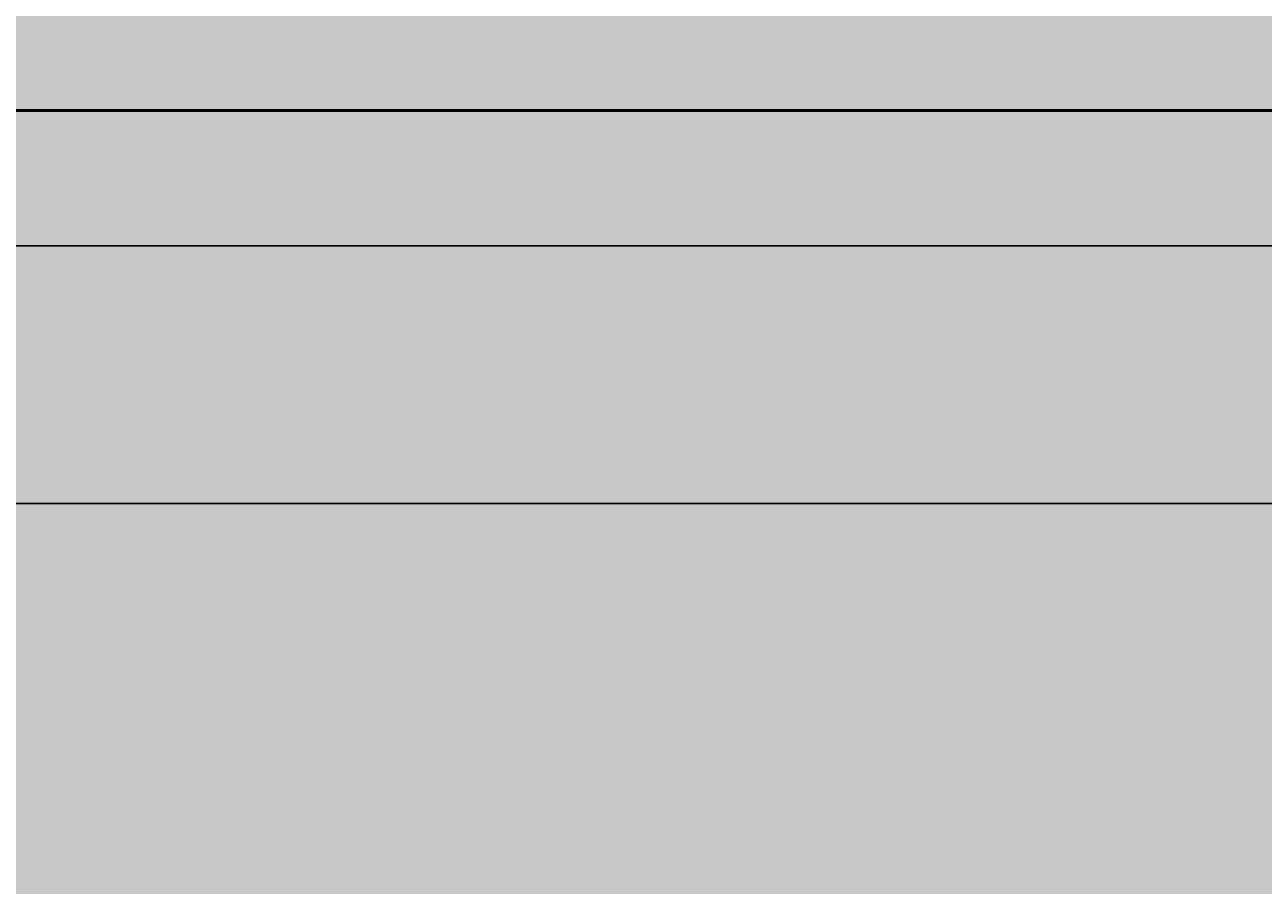
# Model space of a CAD drawing. Units: inches. Extents: x -12 to 334, y -10 to 186.
# Tile 43 of 77: x 175 to 198, y 49 to 65. Entities that reach past the tile are written whole.
import ezdxf
from ezdxf import colors
from ezdxf.entities.mleader import LeaderData, LeaderLine
from ezdxf.math import Vec2, Vec3

# ---------------------------------------------------------------- set-up
doc = ezdxf.new("R2010")
doc.units = ezdxf.units.IN
doc.header["$MEASUREMENT"] = 0
for name, color, linetype, lineweight in [('M-ANNO-TEXT', 3, 'Continuous', 25), ('M-DIMS', 2, 'Continuous', 18), ('M-EQPM', 7, 'Continuous', 50), ('M-EQPM-PATT', 8, 'Continuous', 18)]:
    doc.layers.add(name, color=color, linetype=linetype, lineweight=lineweight)
doc.styles.get("Standard").update_dxf_attribs({"font": 'arial.ttf'})
doc.dimstyles.get("Standard").update_dxf_attribs({"dimtxt": 0.18, "dimasz": 0.18, "dimexe": 0.18, "dimexo": 0.0625, "dimgap": 0.09, "dimtad": 0, "dimtih": 1, "dimtoh": 1, "dimdec": 4, "dimzin": 0, "dimdsep": 46, "dimtxsty": 'Standard', "dimcen": 0.09, "dimadec": 0, "dimazin": 0, "dimtfac": 1, "dimtdec": 4, "dimtofl": 0, "dimtmove": 0, "dimatfit": 3, "dimfxl": 1, "dimtolj": 1, "dimtzin": 0, "dimarcsym": 0})

# ---------------------------------------------------------------- blocks, each defined once
blk = doc.blocks.new('*D1')
at = {"layer": 'Defpoints', "color": 0, "transparency": 16777216}
for p in [(281.426, 91.899), (3.376, 80.692), (281.426, 14.304)]:
    blk.add_point(p, dxfattribs=at)
at = {"layer": 'M-DIMS', "color": 0, "lineweight": -2, "transparency": 16777216}
for p, q in [((281.426, 91.836), (281.426, 14.124)), ((3.376, 80.629), (3.376, 14.124)), ((3.556, 14.304), (141.935, 14.304)), ((281.246, 14.304), (142.867, 14.304))]:
    blk.add_line(p, q, dxfattribs=at)
at = {"layer": 'M-DIMS', "color": 0, "transparency": 16777216}
for points in [[(3.556, 14.334), (3.556, 14.274), (3.376, 14.304)], [(281.246, 14.334), (281.246, 14.274), (281.426, 14.304)]]:
    blk.add_solid(points, dxfattribs=at)
at = {"layer": 'M-DIMS', "color": 0, "transparency": 16777216, "insert": (142.401, 14.304), "char_height": 0.18, "attachment_point": 5}
blk.add_mtext('\\A1;278.05', dxfattribs=at)
blk = doc.blocks.new('*D17')
at = {"layer": 'Defpoints', "color": 0, "transparency": 16777216}
for p in [(106.177, 102.896), (105.892, 56.321), (295.976, 56.321)]:
    blk.add_point(p, dxfattribs=at)
at = {"layer": 'M-DIMS', "color": 0, "lineweight": -2, "transparency": 16777216}
for p, q in [((106.24, 102.896), (296.156, 102.896)), ((295.976, 102.716), (295.976, 79.79)), ((295.976, 56.501), (295.976, 79.426)), ((105.954, 56.321), (296.156, 56.321))]:
    blk.add_line(p, q, dxfattribs=at)
at = {"layer": 'M-DIMS', "color": 0, "transparency": 16777216}
for points in [[(295.946, 102.716), (296.006, 102.716), (295.976, 102.896)], [(295.946, 56.501), (296.006, 56.501), (295.976, 56.321)]]:
    blk.add_solid(points, dxfattribs=at)
at = {"layer": 'M-DIMS', "color": 0, "transparency": 16777216, "insert": (295.976, 79.608), "char_height": 0.18, "attachment_point": 5}
blk.add_mtext('\\A1;46.575', dxfattribs=at)
blk = doc.blocks.new('*D32')
at = {"layer": 'Defpoints', "color": 0, "transparency": 16777216}
for p in [(170.908, 61.105), (216.428, 61.105), (216.428, 14.304)]:
    blk.add_point(p, dxfattribs=at)
at = {"layer": 'M-DIMS', "color": 0, "lineweight": -2, "transparency": 16777216}
for p, q in [((170.908, 61.042), (170.908, 14.124)), ((216.428, 61.042), (216.428, 14.124)), ((171.088, 14.304), (193.271, 14.304)), ((216.248, 14.304), (194.064, 14.304))]:
    blk.add_line(p, q, dxfattribs=at)
at = {"layer": 'M-DIMS', "color": 0, "transparency": 16777216}
for points in [[(171.088, 14.334), (171.088, 14.274), (170.908, 14.304)], [(216.248, 14.334), (216.248, 14.274), (216.428, 14.304)]]:
    blk.add_solid(points, dxfattribs=at)
at = {"layer": 'M-DIMS', "color": 0, "transparency": 16777216, "insert": (193.668, 14.304), "char_height": 0.18, "attachment_point": 5}
blk.add_mtext('\\A1;45.52', dxfattribs=at)
blk = doc.blocks.new('*D35')
at = {"layer": 'Defpoints', "color": 0, "transparency": 16777216}
for p in [(216.428, 98.108), (-11.174, 61.105), (216.428, 61.105)]:
    blk.add_point(p, dxfattribs=at)
at = {"layer": 'M-DIMS', "color": 0, "lineweight": -2, "transparency": 16777216}
for p, q in [((216.365, 98.108), (-11.354, 98.108)), ((-11.174, 97.928), (-11.174, 79.788)), ((-11.174, 61.285), (-11.174, 79.424)), ((216.365, 61.105), (-11.354, 61.105))]:
    blk.add_line(p, q, dxfattribs=at)
at = {"layer": 'M-DIMS', "color": 0, "transparency": 16777216}
for points in [[(-11.204, 97.928), (-11.144, 97.928), (-11.174, 98.108)], [(-11.204, 61.285), (-11.144, 61.285), (-11.174, 61.105)]]:
    blk.add_solid(points, dxfattribs=at)
at = {"layer": 'M-DIMS', "color": 0, "transparency": 16777216, "insert": (-11.174, 79.606), "char_height": 0.18, "attachment_point": 5}
blk.add_mtext('\\A1;37', dxfattribs=at)
blk = doc.blocks.new('*D39')
at = {"layer": 'Defpoints', "color": 0, "transparency": 16777216}
for p in [(279.726, 80.692), (-11.174, 45.854), (269.381, 45.854)]:
    blk.add_point(p, dxfattribs=at)
at = {"layer": 'M-DIMS', "color": 0, "lineweight": -2, "transparency": 16777216}
for p, q in [((279.664, 80.692), (-11.354, 80.692)), ((-11.174, 80.512), (-11.174, 63.455)), ((-11.174, 46.034), (-11.174, 63.091)), ((269.318, 45.854), (-11.354, 45.854))]:
    blk.add_line(p, q, dxfattribs=at)
at = {"layer": 'M-DIMS', "color": 0, "transparency": 16777216}
for points in [[(-11.204, 80.512), (-11.144, 80.512), (-11.174, 80.692)], [(-11.204, 46.034), (-11.144, 46.034), (-11.174, 45.854)]]:
    blk.add_solid(points, dxfattribs=at)
at = {"layer": 'M-DIMS', "color": 0, "transparency": 16777216, "insert": (-11.174, 63.273), "char_height": 0.18, "attachment_point": 5}
blk.add_mtext('\\A1;34.84', dxfattribs=at)
blk = doc.blocks.new('*D41')
at = {"layer": 'Defpoints', "color": 0, "transparency": 16777216}
for p in [(190.169, 91.899), (277.343, 68.515)]:
    blk.add_point(p, dxfattribs=at)
at = {"layer": 'M-DIMS', "color": 0, "lineweight": -2, "transparency": 16777216}
for p, q in [((190.169, 91.809), (190.169, 91.989)), ((190.079, 91.899), (190.259, 91.899)), ((329.648, 54.485), (277.517, 68.469)), ((329.828, 54.485), (329.648, 54.485))]:
    blk.add_line(p, q, dxfattribs=at)
at = {"layer": 'M-DIMS', "color": 0, "transparency": 16777216}
blk.add_solid([(277.525, 68.498), (277.509, 68.44), (277.343, 68.515)], dxfattribs=at)
at = {"layer": 'M-DIMS', "color": 0, "transparency": 16777216, "insert": (330.307, 54.485), "char_height": 0.18, "attachment_point": 5}
blk.add_mtext('\\A1;R90.26', dxfattribs=at)

msp = doc.modelspace()

# ---------------------------------------------------------------- hatches: boundary and pattern name
at = {"layer": 'M-EQPM-PATT'}
h = msp.add_hatch(color=256, dxfattribs=at)
h.set_gradient(color1=(205, 32, 39), color2=(205, 32, 39), tint=1)
h.paths.add_polyline_path([(64.5, 80.754), (64.5, 89.8963), (226.6083, 89.8963, -1), (226.6083, 69.6117), (64.5, 69.6117), (64.5, 78.754), (4.4744, 78.754, 0.384914), (23.5807, 61.4872), (37.1002, 61.4872), (37.1002, 33.6752), (53.1002, 33.6752), (53.1002, 61.4872), (64.5, 61.4872), (64.5, 63.6117), (226.6083, 63.6117, 1), (226.6083, 95.8963), (64.5, 95.8963), (64.5, 99.8958), (53.1002, 99.8958), (53.1002, 127.7078), (37.1002, 127.7078), (37.1002, 99.8958), (23.5807, 99.8958, 0.4132606), (4.3766, 80.754)])
h.paths.add_polyline_path([(64.5, 91.8963), (64.5, 93.8963), (226.6083, 93.8963, -1), (226.6083, 65.6117), (64.5, 65.6117), (64.5, 67.6117), (226.6083, 67.6117, 1), (226.6083, 91.8963)], flags=16)
h = msp.add_hatch(color=256, dxfattribs=at)
h.set_gradient(color1=(94, 103, 175), color2=(94, 103, 175), tint=1)
h.paths.add_polyline_path([(129.093, 89.8963), (86.8879, 89.8963), (86.8879, 69.6117), (129.093, 69.6117)], flags=17)
h.paths.add_polyline_path([(170.9079, 89.8963), (130.8573, 89.8963), (130.8573, 69.6117), (170.9079, 69.6117)], flags=17)
h.paths.add_polyline_path([(216.4278, 89.8963), (172.6722, 89.8963), (172.6722, 69.6117), (216.4278, 69.6117)], flags=17)
h.paths.add_polyline_path([(245.9354, 82.6969), (247.9354, 82.6969), (247.9354, 46.8541), (268.3808, 46.8541, 0.0998398), (279.7263, 80.6915), (251.9801, 80.6915, 0.4142136), (231.7758, 100.8958), (84.7229, 100.8958), (84.7229, 109.0583), (83.7229, 109.0583), (83.7229, 95.8963), (129.093, 95.8963), (129.093, 98.1081), (130.8573, 98.1081), (130.8573, 95.8963), (170.9079, 95.8963), (170.9079, 98.1081), (172.6722, 98.1081), (172.6722, 95.8963), (216.4278, 95.8963), (216.4278, 98.1081), (218.1922, 98.1081), (218.1922, 95.8963), (226.6083, 95.8963, -1), (226.6083, 63.6117), (218.1922, 63.6117), (218.1922, 61.1045), (216.4278, 61.1045), (216.4278, 63.6117), (172.6722, 63.6117), (172.6722, 61.1045), (170.9079, 61.1045), (170.9079, 63.6117), (130.8573, 63.6117), (130.8573, 61.1045), (129.093, 61.1045), (129.093, 63.6117), (87.8879, 63.6117), (87.8879, 56.3205), (105.8919, 56.3205), (105.8919, 28.8541), (115.8919, 28.8541), (115.8919, 46.8541), (222.5761, 46.8541), (222.5761, 30.8541), (232.5761, 30.8541), (232.5761, 46.8541), (245.9354, 46.8541)])
h.paths.add_polyline_path([(86.8879, 89.8963), (75.9244, 89.8963), (75.9244, 69.6117), (86.8879, 69.6117)])
h.paths.add_polyline_path([(83.7229, 109.0583), (75.9244, 109.0583), (75.9244, 95.8963), (83.7229, 95.8963)])
h.paths.add_polyline_path([(226.6083, 89.8963), (218.1922, 89.8963), (218.1922, 69.6117), (226.6083, 69.6117, 1)], flags=17)
h = msp.add_hatch(color=256, dxfattribs=at)
h.set_gradient(color1=(0, 0, 255), color2=(0, 0, 255), tint=1)
h.paths.add_polyline_path([(84.7229, 100.8958), (84.7229, 109.0583), (83.7229, 109.0583), (83.7229, 95.8963), (129.093, 95.8963), (129.093, 98.1081), (130.8573, 98.1081), (130.8573, 95.8963), (170.9079, 95.8963), (170.9079, 98.1081), (172.6722, 98.1081), (172.6722, 95.8963), (216.4278, 95.8963), (216.4278, 98.1081), (218.1922, 98.1081), (218.1922, 95.8963), (226.6083, 95.8963, -1), (226.6083, 63.6117), (218.1922, 63.6117), (218.1922, 61.1045), (216.4278, 61.1045), (216.4278, 63.6117), (172.6722, 63.6117), (172.6722, 61.1045), (170.9079, 61.1045), (170.9079, 63.6117), (130.8573, 63.6117), (130.8573, 61.1045), (129.093, 61.1045), (129.093, 63.6117), (87.8879, 63.6117), (87.8879, 56.3205), (105.8919, 56.3205), (105.8919, 28.8541), (115.8919, 28.8541), (115.8919, 46.8541), (222.5761, 46.8541), (222.5761, 30.8541), (232.5761, 30.8541), (232.5761, 46.8541), (245.9354, 46.8541), (245.9354, 82.6969), (247.9354, 82.6969), (247.9354, 46.8541), (268.3808, 46.8541, 0.0998398), (279.7263, 80.6915), (251.9801, 80.6915, 0.4142136), (231.7758, 100.8958)])

# ---------------------------------------------------------------- linework, layer by layer
at = {"layer": 'M-EQPM'}
msp.add_lwpolyline([(64.5, 63.6117), (226.6083, 63.6117, 1), (226.6083, 95.8963), (64.5, 95.8963)], format="xyb", dxfattribs=at)

# ---------------------------------------------------------------- dimensions: what is measured, and where the dimension line sits
at = {"layer": 'M-DIMS'}
for base, p1, p2, override, picture, middle in [((295.9756, 56.3205), (106.1771, 102.8958), (105.8919, 56.3205), {"dimdec": 3, "dimlfac": 1, "dimrnd": 0, "dimzin": 0, "dimdsep": 46, "dimlunit": 2}, '*D17', (295.9756, 79.6082)), ((-11.1736, 61.1045), (216.4278, 98.1081), (216.4278, 61.1045), {"dimdec": 0, "dimlfac": 1, "dimrnd": 0, "dimzin": 0, "dimdsep": 46, "dimlunit": 2}, '*D35', (-11.1735, 79.6063)), ((-11.1736, 45.8541), (279.7263, 80.6915), (269.3808, 45.8541), {"dimdec": 2, "dimlfac": 1, "dimrnd": 0, "dimzin": 0, "dimdsep": 46, "dimlunit": 2}, '*D39', (-11.1735, 63.2728))]:
    dim = msp.add_linear_dim(base=base, p1=p1, p2=p2, angle=90, dimstyle='Standard', override=override, dxfattribs=at)
    dim.commit()
    dim.dimension.update_dxf_attribs({"geometry": picture, "text_midpoint": middle})
dim = msp.add_radius_dim(center=(190.1689, 91.8988), mpoint=(277.3431, 68.5153), dimstyle='Standard', override={"dimdec": 2, "dimlfac": 1, "dimrnd": 0, "dimzin": 0, "dimdsep": 46, "dimlunit": 2}, dxfattribs=at)
dim.commit()
dim.dimension.update_dxf_attribs({"geometry": '*D41', "text_midpoint": (330.3074, 54.4851), "dimtype": 164})
for base, p1, p2, picture, middle in [((281.4256, 14.3041), (3.3765, 80.6915), (281.4256, 91.8988), '*D1', (142.401, 14.3041)), ((216.4278, 14.3041), (170.9079, 61.1045), (216.4278, 61.1045), '*D32', (193.6678, 14.3041))]:
    dim = msp.add_linear_dim(base=base, p1=p1, p2=p2, dimstyle='Standard', override={"dimdec": 2, "dimlfac": 1, "dimrnd": 0, "dimzin": 0, "dimdsep": 46, "dimlunit": 2}, dxfattribs=at)
    dim.commit()
    dim.dimension.update_dxf_attribs({"geometry": picture, "text_midpoint": middle})

# ---------------------------------------------------------------- leaders
at = {"layer": 'M-ANNO-TEXT'}
ml = msp.add_multileader_mtext('Standard', dxfattribs=at)
ml.set_content('u-tubes', color=256)
ml.set_leader_properties()
ml.build(insert=Vec2(0, 0))
ml.multileader.update_dxf_attribs({"dogleg_length": 0.36, "arrow_head_size": 0.7})
ctx = ml.context
ctx.base_point, ctx.arrow_head_size, ctx.landing_gap_size, ctx.plane_origin = Vec3(183.1578, 33.1882), 0.7, 0.09, Vec3(168.0474, 30.6523)
ctx.text_align_type = 2
notes = []
notes.append((ctx, [(1, (1, 1, 0), (206.8598, 33.1882), (-1, 0), 5.4565, [(0, [(213.6735, 63.6117)], 0, [])])]))
ctx.mtext.insert, ctx.mtext.alignment, ctx.mtext.flow_direction = Vec3(201.3133, 35.2209), 3, 5
for ctx, leaders in notes:
    for number, flags, end, landing, length, lines in leaders:
        leader = LeaderData()
        leader.index, (leader.has_last_leader_line, leader.has_dogleg_vector, leader.attachment_direction) = number, flags
        leader.last_leader_point, leader.dogleg_vector, leader.dogleg_length = Vec3(end), Vec3(landing), length
        for number, points, colour, breaks in lines:
            line = LeaderLine()
            line.index, line.vertices, line.color, line.breaks = number, Vec3.list(points), colors.encode_raw_color(colour), breaks
            leader.lines.append(line)
        ctx.leaders.append(leader)

doc.saveas('drawing.dxf')
